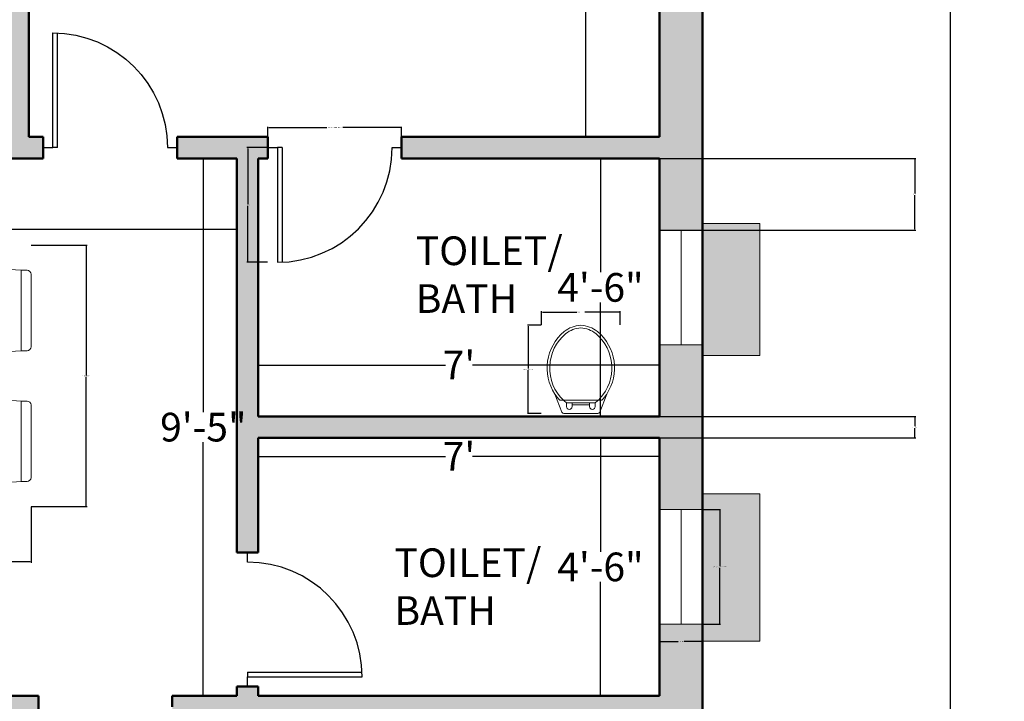
# Model space of a CAD drawing. Units: inches. Extents: x -28 to 544, y -640 to 52.
# Tile 10 of 11: x 338 to 544, y -251 to -109. Entities that reach past the tile are written whole.
import ezdxf

# ---------------------------------------------------------------- set-up
doc = ezdxf.new("R2010")
doc.units = ezdxf.units.IN
doc.header["$MEASUREMENT"] = 0
for name, color, linetype, lineweight in [('A-ANNO-DIMS', 2, 'Continuous', 18), ('A-AREA-IDEN', 7, 'Continuous', 25), ('A-DOOR', 3, 'Continuous', 25), ('A-FLOR-FIXT', 9, 'Continuous', 20), ('A-FURN', 8, 'Continuous', 18), ('A-GLAZ', 4, 'Continuous', 20), ('A-ROOF', 8, 'Continuous', 18), ('A-ROOF-PATT', 252, 'Continuous', 13), ('A-WALL', 7, 'Continuous', 50), ('A-WALL-PATT', 5, 'Continuous', 13)]:
    doc.layers.add(name, color=color, linetype=linetype, lineweight=lineweight)
doc.styles.get("Standard").update_dxf_attribs({"font": 'arial.ttf'})
doc.dimstyles.get("Standard").update_dxf_attribs({"dimtxt": 0.18, "dimasz": 0.18, "dimexe": 0.18, "dimexo": 0.0625, "dimgap": 0.09, "dimtad": 0, "dimtih": 1, "dimtoh": 1, "dimdec": 0, "dimzin": 0, "dimdsep": 46, "dimlunit": 3, "dimtxsty": 'Standard', "dimcen": 0.09, "dimadec": 0, "dimazin": 0, "dimtfac": 1, "dimtdec": 0, "dimtofl": 0, "dimtmove": 0, "dimatfit": 3, "dimfxl": 1, "dimtolj": 1, "dimtzin": 0, "dimarcsym": 0})

# ---------------------------------------------------------------- blocks, each defined once
blk = doc.blocks.new('*D7')
at = {"layer": 'A-ANNO-DIMS', "color": 0, "lineweight": -2, "transparency": 16777216}
for p, q in [((456.03, -1.42), (456.03, -64.14)), ((456.09, -1.24), (456.21, -1.24)), ((456.03, -133.06), (456.03, -70.34)), ((456.09, -133.24), (456.21, -133.24))]:
    blk.add_line(p, q, dxfattribs=at)
at = {"layer": 'A-ANNO-DIMS', "color": 0, "transparency": 16777216}
for points in [[(456, -1.42), (456.06, -1.42), (456.03, -1.24)], [(456, -133.06), (456.06, -133.06), (456.03, -133.24)]]:
    blk.add_solid(points, dxfattribs=at)
at = {"layer": 'Defpoints', "color": 0, "transparency": 16777216}
for p in [(456.03, -1.24), (456.03, -133.24), (456.03, -133.24)]:
    blk.add_point(p, dxfattribs=at)
at = {"layer": 'A-ANNO-DIMS', "color": 0, "transparency": 16777216, "insert": (456.03, -67.24), "char_height": 6, "attachment_point": 5}
blk.add_mtext("\\A1;11'", dxfattribs=at)
blk = doc.blocks.new('*D11')
at = {"layer": 'A-ANNO-DIMS', "color": 0, "lineweight": -2, "transparency": 16777216}
for p, q in [((387.44, -185.36), (387.44, -180.82)), ((387.62, -181), (426.62, -181)), ((471.26, -181), (432.27, -181)), ((471.44, -185.36), (471.44, -180.82))]:
    blk.add_line(p, q, dxfattribs=at)
at = {"layer": 'A-ANNO-DIMS', "color": 0, "transparency": 16777216}
for points in [[(387.62, -180.97), (387.62, -181.03), (387.44, -181)], [(471.26, -180.97), (471.26, -181.03), (471.44, -181)]]:
    blk.add_solid(points, dxfattribs=at)
at = {"layer": 'Defpoints', "color": 0, "transparency": 16777216}
for p in [(471.44, -181), (387.44, -185.42), (471.44, -185.42)]:
    blk.add_point(p, dxfattribs=at)
at = {"layer": 'A-ANNO-DIMS', "color": 0, "transparency": 16777216, "insert": (429.44, -181), "char_height": 6, "attachment_point": 5}
blk.add_mtext("\\A1;7'", dxfattribs=at)
blk = doc.blocks.new('*D12')
at = {"layer": 'A-ANNO-DIMS', "color": 0, "lineweight": -2, "transparency": 16777216}
for p, q in [((459.06, -137.92), (459.06, -161.59)), ((459.12, -137.74), (459.24, -137.74)), ((459.06, -191.56), (459.06, -167.89)), ((459.12, -191.74), (459.24, -191.74))]:
    blk.add_line(p, q, dxfattribs=at)
at = {"layer": 'A-ANNO-DIMS', "color": 0, "transparency": 16777216}
for points in [[(459.03, -137.92), (459.09, -137.92), (459.06, -137.74)], [(459.03, -191.56), (459.09, -191.56), (459.06, -191.74)]]:
    blk.add_solid(points, dxfattribs=at)
at = {"layer": 'Defpoints', "color": 0, "transparency": 16777216}
for p in [(459.06, -137.74), (459.06, -191.74), (459.06, -191.74)]:
    blk.add_point(p, dxfattribs=at)
at = {"layer": 'A-ANNO-DIMS', "color": 0, "transparency": 16777216, "insert": (459.06, -164.74), "char_height": 6, "attachment_point": 5}
blk.add_mtext('\\A1;4\'-6"', dxfattribs=at)
blk = doc.blocks.new('*D17')
at = {"layer": 'A-ANNO-DIMS', "color": 0, "lineweight": -2, "transparency": 16777216}
for p, q in [((459.06, -196.42), (459.06, -220.09)), ((459.12, -196.24), (459.24, -196.24)), ((459.06, -250.06), (459.06, -226.39)), ((459.12, -250.24), (459.24, -250.24))]:
    blk.add_line(p, q, dxfattribs=at)
at = {"layer": 'A-ANNO-DIMS', "color": 0, "transparency": 16777216}
for points in [[(459.03, -196.42), (459.09, -196.42), (459.06, -196.24)], [(459.03, -250.06), (459.09, -250.06), (459.06, -250.24)]]:
    blk.add_solid(points, dxfattribs=at)
at = {"layer": 'Defpoints', "color": 0, "transparency": 16777216}
for p in [(459.06, -196.24), (459.06, -250.24), (459.06, -250.24)]:
    blk.add_point(p, dxfattribs=at)
at = {"layer": 'A-ANNO-DIMS', "color": 0, "transparency": 16777216, "insert": (459.06, -223.24), "char_height": 6, "attachment_point": 5}
blk.add_mtext('\\A1;4\'-6"', dxfattribs=at)
blk = doc.blocks.new('*D18')
at = {"layer": 'A-ANNO-DIMS', "color": 0, "lineweight": -2, "transparency": 16777216}
for p, q in [((387.44, -200.06), (387.44, -199.94)), ((387.62, -200.12), (426.62, -200.12)), ((471.26, -200.12), (432.27, -200.12)), ((471.44, -200.06), (471.44, -199.94))]:
    blk.add_line(p, q, dxfattribs=at)
at = {"layer": 'A-ANNO-DIMS', "color": 0, "transparency": 16777216}
for points in [[(387.62, -200.09), (387.62, -200.15), (387.44, -200.12)], [(471.26, -200.09), (471.26, -200.15), (471.44, -200.12)]]:
    blk.add_solid(points, dxfattribs=at)
at = {"layer": 'Defpoints', "color": 0, "transparency": 16777216}
for p in [(387.44, -200.12), (471.44, -200.12), (471.44, -200.12)]:
    blk.add_point(p, dxfattribs=at)
at = {"layer": 'A-ANNO-DIMS', "color": 0, "transparency": 16777216, "insert": (429.44, -200.12), "char_height": 6, "attachment_point": 5}
blk.add_mtext("\\A1;7'", dxfattribs=at)
blk = doc.blocks.new('*D28')
at = {"layer": 'A-ANNO-DIMS', "color": 0, "lineweight": -2, "transparency": 16777216}
for p, q in [((480.51, 7.76), (532.47, 7.76)), ((532.29, 7.58), (532.29, -286.84)), ((532.29, -587.56), (532.29, -293.14)), ((480.51, -587.74), (532.47, -587.74))]:
    blk.add_line(p, q, dxfattribs=at)
at = {"layer": 'A-ANNO-DIMS', "color": 0, "transparency": 16777216}
for points in [[(532.26, 7.58), (532.32, 7.58), (532.29, 7.76)], [(532.26, -587.56), (532.32, -587.56), (532.29, -587.74)]]:
    blk.add_solid(points, dxfattribs=at)
at = {"layer": 'Defpoints', "color": 0, "transparency": 16777216}
for p in [(480.44, 7.76), (480.44, -587.74), (532.29, -587.74)]:
    blk.add_point(p, dxfattribs=at)
at = {"layer": 'A-ANNO-DIMS', "color": 0, "transparency": 16777216, "insert": (532.29, -289.99), "char_height": 6, "attachment_point": 5}
blk.add_mtext('\\A1;49\'-8"', dxfattribs=at)
blk = doc.blocks.new('*D36')
at = {"layer": 'A-ANNO-DIMS', "color": 0, "lineweight": -2, "transparency": 16777216}
for p, q in [((376.13, -137.74), (375.76, -137.74)), ((375.94, -137.92), (375.94, -190.84)), ((375.94, -250.06), (375.94, -197.14)), ((376.13, -250.24), (375.76, -250.24))]:
    blk.add_line(p, q, dxfattribs=at)
at = {"layer": 'A-ANNO-DIMS', "color": 0, "transparency": 16777216}
for points in [[(375.91, -137.92), (375.97, -137.92), (375.94, -137.74)], [(375.91, -250.06), (375.97, -250.06), (375.94, -250.24)]]:
    blk.add_solid(points, dxfattribs=at)
at = {"layer": 'Defpoints', "color": 0, "transparency": 16777216}
for p in [(375.94, -137.74), (376.19, -137.74), (376.19, -250.24)]:
    blk.add_point(p, dxfattribs=at)
at = {"layer": 'A-ANNO-DIMS', "color": 0, "transparency": 16777216, "insert": (375.94, -193.99), "char_height": 6, "attachment_point": 5}
blk.add_mtext('\\A1;9\'-5"', dxfattribs=at)
blk = doc.blocks.new('*D38')
at = {"layer": 'A-ANNO-DIMS', "color": 0, "lineweight": -2, "transparency": 16777216}
for p, q in [((250.94, -155.24), (250.94, -152.45)), ((382.94, -152.31), (382.94, -152.81)), ((251.12, -152.63), (312.05, -152.63)), ((382.76, -152.63), (321.84, -152.63))]:
    blk.add_line(p, q, dxfattribs=at)
at = {"layer": 'A-ANNO-DIMS', "color": 0, "transparency": 16777216}
for points in [[(251.12, -152.6), (251.12, -152.66), (250.94, -152.63)], [(382.76, -152.6), (382.76, -152.66), (382.94, -152.63)]]:
    blk.add_solid(points, dxfattribs=at)
at = {"layer": 'Defpoints', "color": 0, "transparency": 16777216}
for p in [(382.94, -152.25), (382.94, -152.63), (250.94, -155.3)]:
    blk.add_point(p, dxfattribs=at)
at = {"layer": 'A-ANNO-DIMS', "color": 0, "transparency": 16777216, "insert": (316.94, -152.63), "char_height": 6, "attachment_point": 5}
blk.add_mtext("\\A1;11'", dxfattribs=at)
blk = doc.blocks.new('DINING-SET-4')
for p, q in [((18.79, 50.59), (2.05, 49.45)), ((58.27, 50.59), (75.01, 49.45)), ((0, 33.45), (0, 48.63)), ((0.82, 49.45), (2.05, 49.45)), ((2.05, 32.63), (2.05, 49.45)), ((20.52, 48.95), (20.52, 33.13)), ((56.54, 48.95), (56.54, 33.13)), ((76.24, 49.45), (75.01, 49.45)), ((75.01, 32.63), (75.01, 49.45)), ((77.06, 33.45), (77.06, 48.63)), ((2.05, 32.63), (0.82, 32.63)), ((2.05, 32.63), (18.79, 31.49)), ((75.01, 32.63), (58.27, 31.49)), ((75.01, 32.63), (76.24, 32.63)), ((2.05, 22.09), (18.79, 23.23)), ((75.01, 22.09), (58.27, 23.23)), ((0, 21.27), (0, 6.09)), ((2.05, 22.09), (0.82, 22.09)), ((2.05, 22.09), (2.05, 5.27)), ((20.52, 5.77), (20.52, 21.59)), ((56.54, 5.77), (56.54, 21.59)), ((75.01, 22.09), (76.24, 22.09)), ((75.01, 22.09), (75.01, 5.27)), ((77.06, 21.27), (77.06, 6.09)), ((0.82, 5.27), (2.05, 5.27)), ((18.79, 4.13), (2.05, 5.27)), ((58.27, 4.13), (75.01, 5.27)), ((76.24, 5.27), (75.01, 5.27))]:
    blk.add_line(p, q)
for points in [[(55.63, 0), (21.43, 0), (21.43, 54.72), (55.63, 54.72)], [(53.35, 2.28), (23.71, 2.28), (23.71, 52.44), (53.35, 52.44)]]:
    blk.add_lwpolyline(points, close=True)
for centre, radius, start, end in [((18.88, 48.95), 1.64, 0, 93.1221), ((58.18, 48.95), 1.64, 86.8779, 180), ((0.82, 48.63), 0.821, 90, 180), ((76.24, 48.63), 0.821, 0, 90), ((0.82, 33.45), 0.821, 180, 270), ((18.88, 33.13), 1.64, 266.8779, 0), ((58.18, 33.13), 1.64, 180, 273.1221), ((76.24, 33.45), 0.821, 270, 0), ((18.88, 21.59), 1.64, 0, 93.1221), ((58.18, 21.59), 1.64, 86.8779, 180), ((0.82, 21.27), 0.821, 90, 180), ((76.24, 21.27), 0.821, 0, 90), ((0.82, 6.09), 0.821, 180, 270), ((18.88, 5.77), 1.64, 266.8779, 0), ((58.18, 5.77), 1.64, 180, 273.1221), ((76.24, 6.09), 0.821, 270, 0)]:
    blk.add_arc(centre, radius, start, end)
blk = doc.blocks.new('WC-PLAN')
for p, q in [((3.43, 2.8), (2.65, 2.8)), ((3.43, 2.8), (7.07, 2.8)), ((10.7, 2.8), (7.07, 2.8)), ((11.48, 2.8), (10.7, 2.8))]:
    blk.add_line(p, q)
for points in [[(1.65, 4.07, -0.383919), (3.59, 17.16, -0.163732), (7.07, 18.49, -0.359733)], [(3.43, 2.8, -0.448546), (3.94, 16.74, -0.162618), (7.07, 17.94, -0.470877)], [(12.48, 4.07, 0.383919), (10.54, 17.16, 0.163732), (7.07, 18.49, 0.359733)], [(11.08, 3.18, 0.431639), (10.19, 16.74, 0.162618), (7.07, 17.94, 0.470877)], [(2.65, 2.8, -0.040937), (1.65, 4.07, -0.163732)], [(7.07, 0), (3.53, 0, -0.31031), (3.1, 0.3), (1.65, 4.07, -0.209071)], [(4.07, 2.24, -0.022712), (3.43, 2.8, -0.162618)], [(7.07, 2.24), (4.07, 2.24, -0.476108)], [(4.07, 2.24), (4.07, 1.47, 1), (5.25, 1.47), (5.25, 1.87)], [(7.07, 0), (10.6, 0, 0.31031), (11.03, 0.3), (12.48, 4.07, 0.209071)], [(7.07, 2.24), (10.07, 2.24, 0.022712)], [(10.07, 2.24), (10.07, 1.47, -1), (8.89, 1.47), (8.89, 1.87)], [(10.07, 2.24, 0.022712), (10.7, 2.8, 0.162618)], [(10.7, 2.8, 0.014165), (11.08, 3.18, 0.162618)], [(11.48, 2.8, 0.040937), (12.48, 4.07, 0.163732)]]:
    blk.add_lwpolyline(points, format="xyb")
for points in [[(5.25, 1.87), (5.25, 2.24)], [(8.89, 1.87), (8.89, 2.24)], [(5.25, 1.87), (8.89, 1.87)]]:
    blk.add_lwpolyline(points)
blk = doc.blocks.new('WIN-24IN')
for p, q in [((0, 0), (0, 24)), ((0, 24), (9, 24)), ((4.5, 0), (4.5, 24)), ((9, 24), (9, 0)), ((9, 0), (0, 0))]:
    blk.add_line(p, q)
blk = doc.blocks.new('DOOR-SWING-24IN')
for p, q in [((25, 0), (25, 24)), ((26, 0), (26, 24)), ((2, 0), (0, 0)), ((25, 0), (26, 0)), ((28, 0), (26, 0))]:
    blk.add_line(p, q)
blk.add_arc((26, 0), 24, 90, 180)
blk = doc.blocks.new('*D59')
at = {"layer": 'A-ANNO-DIMS', "color": 0, "lineweight": -2, "transparency": 16777216}
for p, q in [((389.44, -135.43), (389.44, -131.11)), ((389.62, -131.29), (401.76, -131.29)), ((417.26, -131.29), (405.12, -131.29)), ((417.44, -135.43), (417.44, -131.11))]:
    blk.add_line(p, q, dxfattribs=at)
at = {"layer": 'A-ANNO-DIMS', "color": 0, "transparency": 16777216}
for points in [[(389.62, -131.26), (389.62, -131.32), (389.44, -131.29)], [(417.26, -131.26), (417.26, -131.32), (417.44, -131.29)]]:
    blk.add_solid(points, dxfattribs=at)
at = {"layer": 'Defpoints', "color": 0, "transparency": 16777216}
for p in [(389.44, -131.29), (389.44, -135.49), (417.44, -135.49)]:
    blk.add_point(p, dxfattribs=at)
at = {"layer": 'A-ANNO-DIMS', "color": 0, "transparency": 16777216, "insert": (403.44, -131.29), "char_height": 0.18, "attachment_point": 5}
blk.add_mtext('\\A1;INTERIOR DOOR 2\'-4" TYP.', dxfattribs=at)
blk = doc.blocks.new('*D60')
at = {"layer": 'A-ANNO-DIMS', "color": 0, "lineweight": -2, "transparency": 16777216}
for p, q in [((389.38, -135.49), (385.06, -135.49)), ((385.24, -135.67), (385.24, -147.31)), ((385.24, -159.31), (385.24, -147.67)), ((389.38, -159.49), (385.06, -159.49))]:
    blk.add_line(p, q, dxfattribs=at)
at = {"layer": 'A-ANNO-DIMS', "color": 0, "transparency": 16777216}
for points in [[(385.21, -135.67), (385.27, -135.67), (385.24, -135.49)], [(385.21, -159.31), (385.27, -159.31), (385.24, -159.49)]]:
    blk.add_solid(points, dxfattribs=at)
at = {"layer": 'Defpoints', "color": 0, "transparency": 16777216}
for p in [(389.44, -135.49), (385.24, -159.49), (389.44, -159.49)]:
    blk.add_point(p, dxfattribs=at)
at = {"layer": 'A-ANNO-DIMS', "color": 0, "transparency": 16777216, "insert": (385.24, -147.49), "char_height": 0.18, "attachment_point": 5}
blk.add_mtext('\\A1;2\'-0" TYP.', dxfattribs=at)
blk = doc.blocks.new('*D61')
at = {"layer": 'A-ANNO-DIMS', "color": 0, "lineweight": -2, "transparency": 16777216}
for p, q in [((480.51, -211.24), (484.22, -211.24)), ((484.04, -211.42), (484.04, -223.06)), ((484.04, -235.06), (484.04, -223.42)), ((480.51, -235.24), (484.22, -235.24))]:
    blk.add_line(p, q, dxfattribs=at)
at = {"layer": 'A-ANNO-DIMS', "color": 0, "transparency": 16777216}
for points in [[(484.01, -211.42), (484.07, -211.42), (484.04, -211.24)], [(484.01, -235.06), (484.07, -235.06), (484.04, -235.24)]]:
    blk.add_solid(points, dxfattribs=at)
at = {"layer": 'Defpoints', "color": 0, "transparency": 16777216}
for p in [(480.44, -211.24), (480.44, -235.24), (484.04, -235.24)]:
    blk.add_point(p, dxfattribs=at)
at = {"layer": 'A-ANNO-DIMS', "color": 0, "transparency": 16777216, "insert": (484.04, -223.24), "char_height": 0.18, "attachment_point": 5}
blk.add_mtext('\\A1;BATH WINDOW 2\'-0" TYP.', dxfattribs=at)
blk = doc.blocks.new('*D62')
at = {"layer": 'A-ANNO-DIMS', "color": 0, "lineweight": -2, "transparency": 16777216}
for p, q in [((471.44, -235.3), (471.44, -239.02)), ((480.44, -235.3), (480.44, -239.02)), ((471.62, -238.84), (475.31, -238.84)), ((480.26, -238.84), (476.58, -238.84))]:
    blk.add_line(p, q, dxfattribs=at)
at = {"layer": 'A-ANNO-DIMS', "color": 0, "transparency": 16777216}
for points in [[(471.62, -238.81), (471.62, -238.87), (471.44, -238.84)], [(480.26, -238.81), (480.26, -238.87), (480.44, -238.84)]]:
    blk.add_solid(points, dxfattribs=at)
at = {"layer": 'Defpoints', "color": 0, "transparency": 16777216}
for p in [(471.44, -235.24), (480.44, -235.24), (471.44, -238.84)]:
    blk.add_point(p, dxfattribs=at)
at = {"layer": 'A-ANNO-DIMS', "color": 0, "transparency": 16777216, "insert": (475.94, -238.84), "char_height": 0.18, "attachment_point": 5}
blk.add_mtext('\\A1;0\'-9" TYP.', dxfattribs=at)
blk = doc.blocks.new('*D71')
at = {"layer": 'A-ANNO-DIMS', "color": 0, "lineweight": -2, "transparency": 16777216}
for p, q in [((262.82, -210.68), (262.82, -222.36)), ((339.88, -210.68), (339.88, -222.36)), ((263, -222.18), (299.96, -222.18)), ((339.7, -222.18), (302.74, -222.18))]:
    blk.add_line(p, q, dxfattribs=at)
at = {"layer": 'A-ANNO-DIMS', "color": 0, "transparency": 16777216}
for points in [[(263, -222.15), (263, -222.21), (262.82, -222.18)], [(339.7, -222.15), (339.7, -222.21), (339.88, -222.18)]]:
    blk.add_solid(points, dxfattribs=at)
at = {"layer": 'Defpoints', "color": 0, "transparency": 16777216}
for p in [(262.82, -210.62), (339.88, -210.62), (339.88, -222.18)]:
    blk.add_point(p, dxfattribs=at)
at = {"layer": 'A-ANNO-DIMS', "color": 0, "transparency": 16777216, "insert": (301.35, -222.18), "char_height": 0.18, "attachment_point": 5}
blk.add_mtext('\\A1;DINING SET 6\'-5" TYP.', dxfattribs=at)
blk = doc.blocks.new('*D72')
at = {"layer": 'A-ANNO-DIMS', "color": 0, "lineweight": -2, "transparency": 16777216}
for p, q in [((339.94, -155.9), (351.62, -155.9)), ((351.44, -156.08), (351.44, -183.08)), ((351.44, -210.44), (351.44, -183.44)), ((339.94, -210.62), (351.62, -210.62))]:
    blk.add_line(p, q, dxfattribs=at)
at = {"layer": 'A-ANNO-DIMS', "color": 0, "transparency": 16777216}
for points in [[(351.41, -156.08), (351.47, -156.08), (351.44, -155.9)], [(351.41, -210.44), (351.47, -210.44), (351.44, -210.62)]]:
    blk.add_solid(points, dxfattribs=at)
at = {"layer": 'Defpoints', "color": 0, "transparency": 16777216}
for p in [(339.88, -155.9), (351.44, -155.9), (339.88, -210.62)]:
    blk.add_point(p, dxfattribs=at)
at = {"layer": 'A-ANNO-DIMS', "color": 0, "transparency": 16777216, "insert": (351.44, -183.26), "char_height": 0.18, "attachment_point": 5}
blk.add_mtext('\\A1;4\'-6 1/2" TYP.', dxfattribs=at)
blk = doc.blocks.new('*D75')
at = {"layer": 'A-ANNO-DIMS', "color": 0, "lineweight": -2, "transparency": 16777216}
for p, q in [((446.68, -172.67), (443.79, -172.67)), ((443.97, -172.85), (443.97, -181.73)), ((443.97, -190.98), (443.97, -182.1)), ((446.68, -191.16), (443.79, -191.16))]:
    blk.add_line(p, q, dxfattribs=at)
at = {"layer": 'A-ANNO-DIMS', "color": 0, "transparency": 16777216}
for points in [[(443.94, -172.85), (444, -172.85), (443.97, -172.67)], [(443.94, -190.98), (444, -190.98), (443.97, -191.16)]]:
    blk.add_solid(points, dxfattribs=at)
at = {"layer": 'Defpoints', "color": 0, "transparency": 16777216}
for p in [(443.97, -172.67), (446.74, -172.67), (446.74, -191.16)]:
    blk.add_point(p, dxfattribs=at)
at = {"layer": 'A-ANNO-DIMS', "color": 0, "transparency": 16777216, "insert": (443.97, -181.92), "char_height": 0.18, "attachment_point": 5}
blk.add_mtext('\\A1;WC 1\'-6 1/2" TYP.', dxfattribs=at)
blk = doc.blocks.new('*D76')
at = {"layer": 'A-ANNO-DIMS', "color": 0, "lineweight": -2, "transparency": 16777216}
for p, q in [((446.74, -172.61), (446.74, -169.72)), ((446.92, -169.9), (454.12, -169.9)), ((462.99, -169.9), (455.8, -169.9)), ((463.17, -172.61), (463.17, -169.72))]:
    blk.add_line(p, q, dxfattribs=at)
at = {"layer": 'A-ANNO-DIMS', "color": 0, "transparency": 16777216}
for points in [[(446.92, -169.87), (446.92, -169.93), (446.74, -169.9)], [(462.99, -169.87), (462.99, -169.93), (463.17, -169.9)]]:
    blk.add_solid(points, dxfattribs=at)
at = {"layer": 'Defpoints', "color": 0, "transparency": 16777216}
for p in [(463.17, -169.9), (446.74, -172.67), (463.17, -172.67)]:
    blk.add_point(p, dxfattribs=at)
at = {"layer": 'A-ANNO-DIMS', "color": 0, "transparency": 16777216, "insert": (454.96, -169.9), "char_height": 0.18, "attachment_point": 5}
blk.add_mtext('\\A1;1\'-4 1/2" TYP.', dxfattribs=at)
blk = doc.blocks.new('*D84')
at = {"layer": 'A-ANNO-DIMS', "color": 0, "lineweight": -2, "transparency": 16777216}
for p, q in [((471.51, -191.74), (525.05, -191.74)), ((524.87, -191.92), (524.87, -193.81)), ((524.87, -196.06), (524.87, -194.17)), ((471.51, -196.24), (525.05, -196.24))]:
    blk.add_line(p, q, dxfattribs=at)
at = {"layer": 'A-ANNO-DIMS', "color": 0, "transparency": 16777216}
for points in [[(524.84, -191.92), (524.9, -191.92), (524.87, -191.74)], [(524.84, -196.06), (524.9, -196.06), (524.87, -196.24)]]:
    blk.add_solid(points, dxfattribs=at)
at = {"layer": 'Defpoints', "color": 0, "transparency": 16777216}
for p in [(471.44, -191.74), (471.44, -196.24), (524.87, -196.24)]:
    blk.add_point(p, dxfattribs=at)
at = {"layer": 'A-ANNO-DIMS', "color": 0, "transparency": 16777216, "insert": (524.87, -193.99), "char_height": 0.18, "attachment_point": 5}
blk.add_mtext('\\A1;0\'-4 1/2"', dxfattribs=at)
blk = doc.blocks.new('*D85')
at = {"layer": 'A-ANNO-DIMS', "color": 0, "lineweight": -2, "transparency": 16777216}
for p, q in [((471.51, -137.74), (525.05, -137.74)), ((524.87, -137.92), (524.87, -145.06)), ((524.87, -152.56), (524.87, -145.42)), ((471.51, -152.74), (525.05, -152.74))]:
    blk.add_line(p, q, dxfattribs=at)
at = {"layer": 'A-ANNO-DIMS', "color": 0, "transparency": 16777216}
for points in [[(524.84, -137.92), (524.9, -137.92), (524.87, -137.74)], [(524.84, -152.56), (524.9, -152.56), (524.87, -152.74)]]:
    blk.add_solid(points, dxfattribs=at)
at = {"layer": 'Defpoints', "color": 0, "transparency": 16777216}
for p in [(471.44, -137.74), (471.44, -152.74), (524.87, -152.74)]:
    blk.add_point(p, dxfattribs=at)
at = {"layer": 'A-ANNO-DIMS', "color": 0, "transparency": 16777216, "insert": (524.87, -145.24), "char_height": 0.18, "attachment_point": 5}
blk.add_mtext('\\A1;1\'-3"', dxfattribs=at)

msp = doc.modelspace()

# ---------------------------------------------------------------- hatches: boundary and pattern name
at = {"layer": 'A-ROOF-PATT'}
h = msp.add_hatch(color=256, dxfattribs=at)
h.dxf.hatch_style = 1
h.set_gradient(color1=(241, 235, 31), color2=(248, 153, 30))
h.paths.add_polyline_path([(124.53, 19.76), (58.75, 19.76), (58.75, 7.76), (124.53, 7.76)])
h.paths.add_polyline_path([(226.33, 19.76), (182.83, 19.76), (182.83, 7.76), (226.33, 7.76)])
h.paths.add_polyline_path([(313.67, 19.76), (271.84, 19.76), (271.84, 7.76), (313.67, 7.76)])
h.paths.add_polyline_path([(440.55, 19.76), (372.16, 19.76), (372.16, 7.76), (440.55, 7.76)])
h.paths.add_polyline_path([(492.44, -34.91), (480.44, -34.91), (480.44, -100.18), (492.44, -100.18)])
h.paths.add_polyline_path([(492.44, -151.37), (480.44, -151.37), (480.44, -179.02), (492.44, -179.02)])
h.paths.add_polyline_path([(492.44, -207.96), (480.44, -207.96), (480.44, -238.77), (492.44, -238.77)])
h.paths.add_polyline_path([(492.44, -289.99), (480.44, -289.99), (480.44, -354.53), (492.44, -354.53)])
h.paths.add_polyline_path([(492.44, -399.27), (480.44, -399.27), (480.44, -430), (492.44, -430)])
h.paths.add_polyline_path([(492.44, -475.99), (480.44, -475.99), (480.44, -546.14), (492.44, -546.14)])
h.paths.add_polyline_path([(442.7, -587.74), (368.43, -587.74), (368.43, -599.74), (442.7, -599.74)])
h.paths.add_polyline_path([(127.64, -587.74), (54.75, -587.74), (54.75, -599.74), (127.64, -599.74)])
h.paths.add_polyline_path([(16.94, -477.43), (4.94, -477.43), (4.94, -547.54), (16.94, -547.54)])
h.paths.add_polyline_path([(16.94, -399.8), (4.94, -399.8), (4.94, -430.58), (16.94, -430.58)])
h.paths.add_polyline_path([(16.94, -287.93), (4.94, -287.93), (4.94, -356.82), (16.94, -356.82)])
h.paths.add_polyline_path([(16.94, -208.93), (4.94, -208.93), (4.94, -240.18), (16.94, -240.18)])
h.paths.add_polyline_path([(16.94, -150), (4.94, -150), (4.94, -180.17), (16.94, -180.17)])
h.paths.add_polyline_path([(16.94, -32.89), (4.94, -32.89), (4.94, -101.73), (16.94, -101.73)])
at = {"layer": 'A-WALL-PATT'}
h = msp.add_hatch(color=256, dxfattribs=at)
h.dxf.hatch_style = 1
h.paths.add_polyline_path([(375.44, 7.76), (310.94, 7.76), (310.94, -1.24), (334.94, -1.24), (334.94, -133.24), (286.94, -133.24), (286.94, -137.74), (342.44, -137.74), (342.44, -133.24), (339.44, -133.24), (339.44, -1.24), (375.44, -1.24)])
h.paths.add_polyline_path([(480.44, 7.76), (435.44, 7.76), (435.44, -1.24), (471.44, -1.24), (471.44, -37.24), (480.44, -37.24)])
h.paths.add_polyline_path([(480.44, -97.24), (471.44, -97.24), (471.44, -133.24), (417.44, -133.24), (417.44, -135.49), (417.44, -137.74), (471.44, -137.74), (471.44, -152.74), (480.44, -152.74)])
h.paths.add_polyline_path([(480.44, -176.74), (471.44, -176.74), (471.44, -191.74), (387.44, -191.74), (387.44, -137.74), (389.44, -137.74), (389.44, -133.24), (370.44, -133.24), (370.44, -135.49), (370.44, -137.74), (382.94, -137.74), (382.94, -191.74), (382.94, -196.24), (382.94, -220.24), (385.19, -220.24), (387.44, -220.24), (387.44, -196.24), (471.44, -196.24), (471.44, -211.24), (480.44, -211.24)])
h.paths.add_polyline_path([(480.44, -235.24), (471.44, -235.24), (471.44, -250.24), (387.44, -250.24), (387.44, -248.24), (382.94, -248.24), (382.94, -250.24), (369.44, -250.24), (369.44, -252.49), (369.44, -254.74), (471.44, -254.74), (471.44, -290.74), (480.44, -290.74)])
h.paths.add_polyline_path([(480.44, -350.74), (471.44, -350.74), (471.44, -386.74), (339.44, -386.74), (339.44, -254.74), (341.44, -254.74), (341.44, -250.24), (334.94, -250.24), (334.94, -391.24), (471.44, -391.24), (471.44, -403.24), (480.44, -403.24)])
h.paths.add_polyline_path([(480.44, -427.24), (471.44, -427.24), (471.44, -439.24), (334.94, -439.24), (334.94, -446.74), (339.44, -446.74), (339.44, -443.74), (471.44, -443.74), (471.44, -481.24), (480.44, -481.24)])
h.paths.add_polyline_path([(480.44, -541.24), (471.44, -541.24), (471.44, -578.74), (435.44, -578.74), (435.44, -587.74), (480.44, -587.74)])
h.paths.add_polyline_path([(375.44, -578.74), (339.44, -578.74), (339.44, -474.74), (337.19, -474.74), (334.94, -474.74), (334.94, -578.74), (296.69, -578.74), (296.69, -587.74), (375.44, -587.74)])

# ---------------------------------------------------------------- linework, layer by layer
at = {"layer": 'A-ROOF'}
for p, q in [((480.44, -151.37), (492.44, -151.37)), ((492.44, -151.37), (492.44, -179.02)), ((492.44, -179.02), (480.44, -179.02)), ((480.44, -207.96), (492.44, -207.96)), ((492.44, -207.96), (492.44, -238.77)), ((492.44, -238.77), (480.44, -238.77))]:
    msp.add_line(p, q, dxfattribs=at)
at = {"layer": 'A-WALL'}
for p, q in [((480.44, 7.76), (480.44, -587.74)), ((339.44, -1.24), (339.44, -133.24)), ((471.44, -1.24), (471.44, -133.24)), ((339.44, -133.24), (342.44, -133.24)), ((342.44, -133.24), (342.44, -137.74)), ((370.44, -135.49), (370.44, -133.24)), ((370.44, -133.24), (389.44, -133.24)), ((389.44, -137.74), (389.44, -133.24)), ((417.44, -135.49), (417.44, -133.24)), ((417.44, -133.24), (471.44, -133.24)), ((370.44, -135.49), (370.44, -137.74)), ((417.44, -135.49), (417.44, -137.74)), ((286.94, -137.74), (342.44, -137.74)), ((370.44, -137.74), (382.94, -137.74)), ((382.94, -137.74), (382.94, -191.74)), ((387.44, -137.74), (387.44, -191.74)), ((387.44, -137.74), (389.44, -137.74)), ((417.44, -137.74), (471.44, -137.74)), ((471.44, -137.74), (471.44, -191.74)), ((382.94, -191.74), (382.94, -196.24)), ((387.44, -191.74), (471.44, -191.74)), ((382.94, -196.24), (382.94, -220.24)), ((387.44, -196.24), (387.44, -220.24)), ((387.44, -196.24), (471.44, -196.24)), ((471.44, -196.24), (471.44, -250.24)), ((385.19, -220.24), (382.94, -220.24)), ((385.19, -220.24), (387.44, -220.24)), ((387.44, -248.24), (382.94, -248.24)), ((382.94, -248.24), (382.94, -250.24)), ((387.44, -248.24), (387.44, -250.24)), ((334.94, -250.24), (341.44, -250.24)), ((341.44, -254.74), (341.44, -250.24)), ((369.44, -252.49), (369.44, -250.24)), ((369.44, -250.24), (382.94, -250.24)), ((387.44, -250.24), (471.44, -250.24))]:
    msp.add_line(p, q, dxfattribs=at)

# ---------------------------------------------------------------- block references
at = {"layer": 'A-DOOR', "extrusion": (0, 0, -1), "zscale": -1}
msp.add_blockref('DOOR-SWING-24IN', (-370.44, -135.49), dxfattribs=at)
at = {"layer": 'A-DOOR'}
for p, rotation in [((417.44, -135.49), 180), ((385.19, -220.24), 270)]:
    msp.add_blockref('DOOR-SWING-24IN', p, dxfattribs=dict(at, rotation=rotation))
at = {"layer": 'A-FLOR-FIXT'}
msp.add_blockref('WC-PLAN', (447.89, -191.16), dxfattribs=at)
at = {"layer": 'A-FURN'}
msp.add_blockref('DINING-SET-4', (262.82, -210.62), dxfattribs=at)
at = {"layer": 'A-GLAZ', "rotation": 180}
for p in [(480.44, -152.74), (480.44, -211.24)]:
    msp.add_blockref('WIN-24IN', p, dxfattribs=at)

# ---------------------------------------------------------------- texts
at = {"layer": 'A-AREA-IDEN', "char_height": 6, "attachment_point": 1}
for insert in [(420.41, -154.08), (415.94, -219.37)]:
    msp.add_mtext('TOILET/\\PBATH', dxfattribs=dict(at, insert=insert))

# ---------------------------------------------------------------- dimensions: what is measured, and where the dimension line sits
at = {"layer": 'A-ANNO-DIMS'}
for base, p1, p2, override, picture, middle in [((532.28608123, -587.74117838), (480.44473605, 7.75882162), (480.44473605, -587.74117838), {"dimtxt": 6, "dimclrd": 0, "dimclre": 0, "dimclrt": 0}, '*D28', (532.28608123, -289.99117838)), ((456.03, -133.24), (456.03, -1.24), (456.03, -133.24), {"dimtxt": 6, "dimclrd": 0, "dimclre": 0, "dimclrt": 0}, '*D7', (456.03, -67.24)), ((375.94450701, -137.74117838), (376.19473605, -250.24117838), (376.19473605, -137.74117838), {"dimtxt": 6, "dimclrd": 0, "dimclre": 0, "dimclrt": 0}, '*D36', (375.94450701, -193.99117838)), ((459.06, -191.74), (459.06, -137.74), (459.06, -191.74), {"dimtxt": 6, "dimclrd": 0, "dimclre": 0, "dimclrt": 0}, '*D12', (459.06, -164.74)), ((524.87, -152.74), (471.44, -137.74), (471.44, -152.74), {"dimdec": 1, "dimlfac": 1, "dimrnd": 0, "dimzin": 1, "dimdsep": 46, "dimlunit": 4, "dimfrac": 2}, '*D85', (524.87, -145.24)), ((524.87, -196.24), (471.44, -191.74), (471.44, -196.24), {"dimdec": 1, "dimlfac": 1, "dimrnd": 0, "dimzin": 1, "dimdsep": 46, "dimlunit": 4, "dimfrac": 2}, '*D84', (524.87, -193.99)), ((459.06, -250.24), (459.06, -196.24), (459.06, -250.24), {"dimtxt": 6, "dimclrd": 0, "dimclre": 0, "dimclrt": 0}, '*D17', (459.06, -223.24))]:
    dim = msp.add_linear_dim(base=base, p1=p1, p2=p2, angle=90, dimstyle='Standard', override=override, dxfattribs=at)
    dim.commit()
    dim.dimension.update_dxf_attribs({"geometry": picture, "text_midpoint": middle})
for base, p1, p2, angle, text, picture, middle in [((389.44, -131.29), (417.44, -135.49), (389.44, -135.49), 180, 'INTERIOR DOOR <> TYP.', '*D59', (403.44, -131.29)), ((385.24, -159.49), (389.44, -135.49), (389.44, -159.49), 270, '<> TYP.', '*D60', (385.24, -147.49)), ((351.44, -155.9), (339.88, -210.62), (339.88, -155.9), 90, '<> TYP.', '*D72', (351.44, -183.26)), ((443.97, -172.67), (446.74, -191.16), (446.74, -172.67), 90, 'WC <> TYP.', '*D75', (443.97, -181.92)), ((484.04, -235.24), (480.44, -211.24), (480.44, -235.24), 270, 'BATH WINDOW <> TYP.', '*D61', (484.04, -223.24)), ((471.44, -238.84), (480.44, -235.24), (471.44, -235.24), 180, '<> TYP.', '*D62', (475.94, -238.84))]:
    dim = msp.add_linear_dim(base=base, p1=p1, p2=p2, angle=angle, text=text, dimstyle='Standard', override={"dimdec": 1, "dimlfac": 1, "dimrnd": 0, "dimzin": 1, "dimdsep": 46, "dimlunit": 4, "dimfrac": 2}, dxfattribs=at)
    dim.commit()
    dim.dimension.update_dxf_attribs({"geometry": picture, "text_midpoint": middle})
for base, p1, p2, picture, middle in [((382.94, -152.63), (250.94, -155.3), (382.94, -152.25), '*D38', (316.94, -152.63)), ((471.44, -181), (387.44, -185.42), (471.44, -185.42), '*D11', (429.44, -181)), ((471.44, -200.12), (387.44, -200.12), (471.44, -200.12), '*D18', (429.44, -200.12))]:
    dim = msp.add_linear_dim(base=base, p1=p1, p2=p2, dimstyle='Standard', override={"dimtxt": 6, "dimclrd": 0, "dimclre": 0, "dimclrt": 0}, dxfattribs=at)
    dim.commit()
    dim.dimension.update_dxf_attribs({"geometry": picture, "text_midpoint": middle})
for base, p1, p2, text, picture, middle in [((463.17, -169.9), (446.74, -172.67), (463.17, -172.67), '<> TYP.', '*D76', (454.96, -169.9)), ((339.88, -222.18), (262.82, -210.62), (339.88, -210.62), 'DINING SET <> TYP.', '*D71', (301.35, -222.18))]:
    dim = msp.add_linear_dim(base=base, p1=p1, p2=p2, text=text, dimstyle='Standard', override={"dimdec": 1, "dimlfac": 1, "dimrnd": 0, "dimzin": 1, "dimdsep": 46, "dimlunit": 4, "dimfrac": 2}, dxfattribs=at)
    dim.commit()
    dim.dimension.update_dxf_attribs({"geometry": picture, "text_midpoint": middle})

doc.saveas('drawing.dxf')
